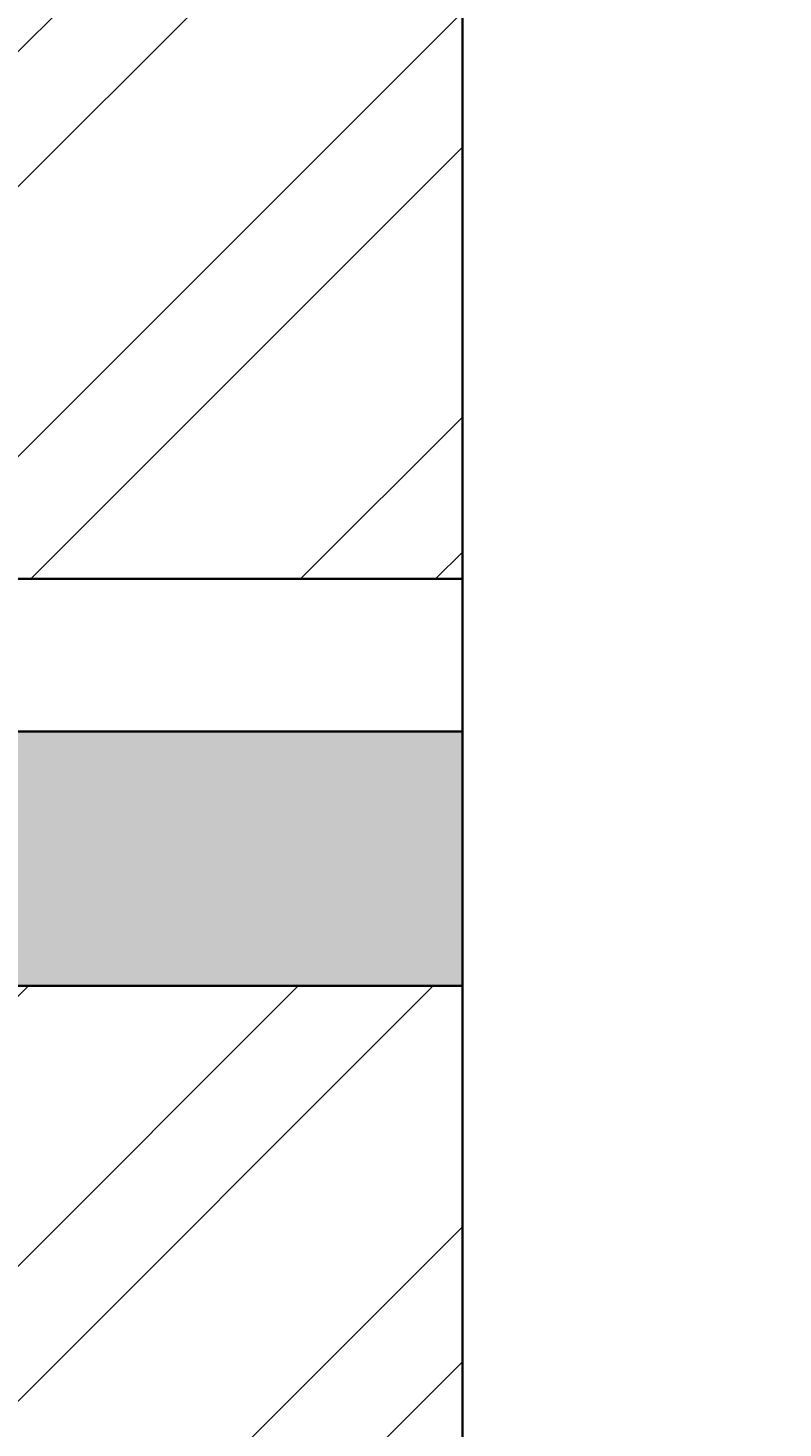
# Model space of a CAD drawing. Units: inches. Extents: x -301 to 715, y -607 to 364.
# Tile 48 of 141: x 135 to 150, y -370 to -343. Entities that reach past the tile are written whole.
import ezdxf

# ---------------------------------------------------------------- set-up
doc = ezdxf.new("R2010")
doc.units = ezdxf.units.IN
doc.header["$MEASUREMENT"] = 0
for name, color, linetype, lineweight in [('A-ANNO-DIMS', 2, 'Continuous', 18), ('A-SECT', 1, 'Continuous', 35), ('A-SECT-PATT', 8, 'Continuous', 13)]:
    doc.layers.add(name, color=color, linetype=linetype, lineweight=lineweight)
doc.styles.get("Standard").update_dxf_attribs({"font": 'arial.ttf'})
doc.dimstyles.get("Standard").update_dxf_attribs({"dimtxt": 0.18, "dimasz": 0.18, "dimexe": 0.18, "dimexo": 0.0625, "dimgap": 0.09, "dimtad": 0, "dimtih": 1, "dimtoh": 1, "dimdec": 1, "dimzin": 0, "dimdsep": 46, "dimlunit": 4, "dimtxsty": 'Standard', "dimcen": 0.09, "dimclrd": 3, "dimclre": 4, "dimclrt": 6, "dimadec": 0, "dimazin": 0, "dimtfac": 1, "dimtdec": 1, "dimtofl": 0, "dimtmove": 0, "dimatfit": 3, "dimfxl": 1, "dimtfill": 2, "dimtfillclr": 51, "dimtolj": 1, "dimtzin": 0, "dimarcsym": 0})

# ---------------------------------------------------------------- blocks, each defined once
blk = doc.blocks.new('*D176')
at = {"layer": 'A-ANNO-DIMS', "color": 4, "lineweight": -2, "transparency": 16777216}
for p, q in [((148.28, -324.477), (215.605, -324.477)), ((-15.22, -540.477), (215.605, -540.477))]:
    blk.add_line(p, q, dxfattribs=at)
at = {"layer": 'A-ANNO-DIMS', "color": 3, "lineweight": -2, "transparency": 16777216}
for p, q in [((215.425, -324.657), (215.425, -432.296)), ((215.425, -540.297), (215.425, -432.659))]:
    blk.add_line(p, q, dxfattribs=at)
at = {"layer": 'A-ANNO-DIMS', "color": 3, "transparency": 16777216}
for points in [[(215.395, -324.657), (215.455, -324.657), (215.425, -324.477)], [(215.395, -540.297), (215.455, -540.297), (215.425, -540.477)]]:
    blk.add_solid(points, dxfattribs=at)
at = {"layer": 'Defpoints', "color": 0, "transparency": 16777216}
for p in [(148.218, -324.477), (-15.282, -540.477), (215.425, -540.477)]:
    blk.add_point(p, dxfattribs=at)
at = {"layer": 'A-ANNO-DIMS', "color": 6, "transparency": 16777216, "insert": (215.425, -432.477), "char_height": 0.18, "attachment_point": 5, "bg_fill": 1, "box_fill_scale": 1.25, "bg_fill_color": 51, "bg_fill_transparency": 0}
blk.add_mtext('\\A1;18\'-0"', dxfattribs=at)
blk = doc.blocks.new('*D186')
at = {"layer": 'A-ANNO-DIMS', "color": 4, "lineweight": -2, "transparency": 16777216}
for p, q in [((134.255, -353.415), (134.255, -292.467)), ((143.218, -353.415), (143.218, -292.467))]:
    blk.add_line(p, q, dxfattribs=at)
at = {"layer": 'A-ANNO-DIMS', "color": 3, "lineweight": -2, "transparency": 16777216}
for p, q in [((134.435, -292.647), (138.407, -292.647)), ((143.038, -292.647), (139.066, -292.647))]:
    blk.add_line(p, q, dxfattribs=at)
at = {"layer": 'A-ANNO-DIMS', "color": 3, "transparency": 16777216}
for points in [[(134.435, -292.617), (134.435, -292.677), (134.255, -292.647)], [(143.038, -292.617), (143.038, -292.677), (143.218, -292.647)]]:
    blk.add_solid(points, dxfattribs=at)
at = {"layer": 'Defpoints', "color": 0, "transparency": 16777216}
for p in [(143.218, -292.647), (134.255, -353.477), (143.218, -353.477)]:
    blk.add_point(p, dxfattribs=at)
at = {"layer": 'A-ANNO-DIMS', "color": 6, "transparency": 16777216, "insert": (138.737, -292.647), "char_height": 0.18, "attachment_point": 5, "bg_fill": 1, "box_fill_scale": 1.25, "bg_fill_color": 51, "bg_fill_transparency": 0}
blk.add_mtext('\\A1;0\'-9"', dxfattribs=at)

msp = doc.modelspace()

# ---------------------------------------------------------------- hatches: boundary and pattern name
at = {"layer": 'A-SECT-PATT'}
h = msp.add_hatch(dxfattribs=at)
h.set_pattern_fill('ANSI32', color=256, scale=15)
h.set_pattern_definition([(45, (10.321, 33.8764), (-3.977476, 3.977476), []), (45, (12.973, 33.8764), (-3.977476, 3.977476), [])])
h.paths.add_polyline_path([(-185.282, -324.477), (-199.282, -324.477), (-199.282, -329.477), (-194.282, -329.477), (-194.282, -353.477), (-185.282, -353.477)])
h.paths.add_polyline_path([(-185.282, -361.477), (-193.904, -361.477), (-193.982, -377.537), (-185.282, -377.537)])
h.paths.add_polyline_path([(143.218, -329.477), (148.218, -329.477), (148.218, -324.477), (134.255, -324.477), (134.255, -353.477), (143.218, -353.477)])
h.paths.add_polyline_path([(143.218, -361.477), (134.255, -361.477), (134.255, -377.477), (143.218, -377.477)])
h.paths.add_polyline_path([(-185.282, -439.477), (-194.282, -439.477), (-194.282, -463.477), (-185.282, -463.477)])
h.paths.add_polyline_path([(-185.282, -471.477), (-194.282, -471.477), (-194.282, -481.477), (-185.282, -481.477)])
h.paths.add_polyline_path([(-185.282, -463.477), (-194.282, -463.477), (-194.282, -466.477), (-185.282, -466.477)])
h.paths.add_polyline_path([(-185.282, -466.477), (-194.282, -466.477), (-194.282, -471.477), (-185.282, -471.477)])
h.paths.add_polyline_path([(-180.282, -481.477), (-185.282, -481.477), (-194.282, -481.477), (-199.282, -481.477), (-199.282, -493.477), (-180.282, -493.477)])
h.paths.add_polyline_path([(-175.282, -493.477), (-180.282, -493.477), (-199.282, -493.477), (-204.282, -493.477), (-204.282, -511.477), (-175.282, -511.477)])
h.paths.add_polyline_path([(-170.282, -511.477), (-175.282, -511.477), (-204.282, -511.477), (-209.282, -511.477), (-209.282, -535.477), (-170.282, -535.477)])
h.paths.add_polyline_path([(-35.282, -463.477), (-41.282, -463.477), (-41.282, -466.477), (-35.282, -466.477)])
h.paths.add_polyline_path([(-35.282, -466.477), (-41.282, -466.477), (-41.282, -471.477), (-35.282, -471.477)])
h.paths.add_polyline_path([(-35.282, -471.477), (-41.282, -471.477), (-41.282, -481.477), (-35.282, -481.477)])
h.paths.add_polyline_path([(-30.282, -481.477), (-46.282, -481.477), (-46.282, -493.477), (-30.282, -493.477)])
h.paths.add_polyline_path([(-25.282, -493.477), (-30.282, -493.477), (-46.282, -493.477), (-51.282, -493.477), (-51.282, -511.477), (-25.282, -511.477)])
h.paths.add_polyline_path([(-20.282, -511.477), (-25.282, -511.477), (-51.282, -511.477), (-56.282, -511.477), (-56.282, -535.477), (-20.282, -535.477)])
h.paths.add_polyline_path([(143.218, -463.477), (134.255, -463.477), (134.255, -466.477), (143.218, -466.477)])
h.paths.add_polyline_path([(143.218, -466.477), (134.255, -466.477), (134.255, -471.477), (143.218, -471.477)])
h.paths.add_polyline_path([(143.218, -471.477), (134.255, -471.477), (134.255, -481.477), (143.218, -481.477)])
h.paths.add_polyline_path([(148.255, -481.477), (143.255, -481.477), (134.255, -481.477), (129.255, -481.477), (129.255, -493.477), (148.255, -493.477)])
h.paths.add_polyline_path([(153.255, -493.477), (148.255, -493.477), (129.255, -493.477), (124.255, -493.477), (124.255, -511.477), (153.255, -511.477)])
h.paths.add_polyline_path([(158.255, -511.477), (153.255, -511.477), (124.255, -511.477), (119.255, -511.477), (119.255, -535.477), (158.255, -535.477)])
h = msp.add_hatch(dxfattribs=at)
h.set_pattern_fill('AR-CONC', color=256, scale=0.5)
h.set_pattern_definition([(50, (10.3213, 33.8764), (3.586301, -0.31376), [0.375, -4.125]), (355, (10.3213, 33.8764), (-0.693757, 3.76096), [0.3, -3.3]), (100.45144, (10.62, 33.8502), (2.892544, 3.4472), [0.3187, -3.50571]), (46.1842, (10.3213, 34.8764), (5.336207, -0.827596), [0.5625, -6.1875]), (96.6356, (10.766, 34.8074), (4.67331, 4.870593), [0.47805, -5.25857]), (351.1842, (10.321, 34.8764), (4.67331, 4.870593), [0.45, -4.95]), (21, (10.8213, 34.6264), (2.984535, -2.013094), [0.375, -4.125]), (326, (10.8213, 34.6264), (1.216577, 3.62575), [0.3, -3.3]), (71.45144, (11.07, 34.4586), (4.201112, 1.612656), [0.3187, -3.50571]), (37.5, (10.3213, 33.8764), (0.0607993, 1.6644693), [0, -3.26, 0, -3.35, 0, -3.3125]), (7.5, (10.3213, 33.8764), (1.3153477, 1.9720586), [0, -1.91, 0, -3.185, 0, -1.2625]), (327.5, (9.2063, 33.8764), (2.6691122, -0.1127744), [0, -1.25, 0, -3.9, 0, -5.175]), (317.5, (8.7063, 33.8764), (2.915931, 0.500525), [0, -1.625, 0, -2.59, 0, -3.675])])
h.paths.add_polyline_path([(-56.282, -535.477), (-61.282, -535.477), (-61.282, -540.477), (-15.282, -540.477), (-15.282, -535.477), (-20.282, -535.477)])
h.paths.add_polyline_path([(119.255, -535.477), (114.255, -535.477), (114.255, -540.477), (163.255, -540.477), (163.255, -535.477), (158.255, -535.477)])
h.paths.add_polyline_path([(-206.282, -471.477), (-209.282, -471.477), (-209.282, -481.477), (-206.282, -481.477), (-194.282, -481.477), (-194.282, -471.477)])
h.paths.add_polyline_path([(-41.282, -481.477), (-41.282, -471.477), (-185.282, -471.477), (-185.282, -481.477), (-180.282, -481.477)])
h.paths.add_polyline_path([(134.255, -481.477), (134.255, -471.477), (-35.282, -471.477), (-35.282, -481.477), (-30.282, -481.477)])
h.paths.add_polyline_path([(155.218, -481.477), (158.218, -481.477), (158.218, -471.477), (153.218, -471.477), (143.218, -471.477), (143.218, -481.477), (148.255, -481.477)])
h.paths.add_polyline_path([(-193.88, -356.477), (-193.904, -361.477), (143.218, -361.477), (143.218, -356.477)])

# ---------------------------------------------------------------- linework, layer by layer
at = {"layer": 'A-SECT'}
for p, q in [((143.218, -353.477), (143.218, -329.477)), ((-194.282, -353.477), (143.218, -353.477)), ((143.218, -353.477), (143.218, -481.477)), ((-194.282, -356.477), (143.218, -356.477)), ((-194.282, -361.477), (143.218, -361.477))]:
    msp.add_line(p, q, dxfattribs=at)

# ---------------------------------------------------------------- dimensions: what is measured, and where the dimension line sits
at = {"layer": 'A-ANNO-DIMS'}
dim = msp.add_linear_dim(base=(143.218, -292.647), p1=(134.255, -353.477), p2=(143.218, -353.477), dimstyle='Standard', override={"dimdec": 1, "dimlfac": 1, "dimrnd": 0, "dimzin": 1, "dimdsep": 46, "dimlunit": 4, "dimfrac": 2}, dxfattribs=at)
dim.commit()
dim.dimension.update_dxf_attribs({"geometry": '*D186', "text_midpoint": (138.737, -292.647)})
dim = msp.add_linear_dim(base=(215.425, -540.477), p1=(148.218, -324.477), p2=(-15.282, -540.477), angle=90, dimstyle='Standard', override={"dimdec": 1, "dimlfac": 1, "dimrnd": 0, "dimzin": 1, "dimdsep": 46, "dimlunit": 4, "dimfrac": 2}, dxfattribs=at)
dim.commit()
dim.dimension.update_dxf_attribs({"geometry": '*D176', "text_midpoint": (215.425, -432.477)})

doc.saveas('drawing.dxf')
